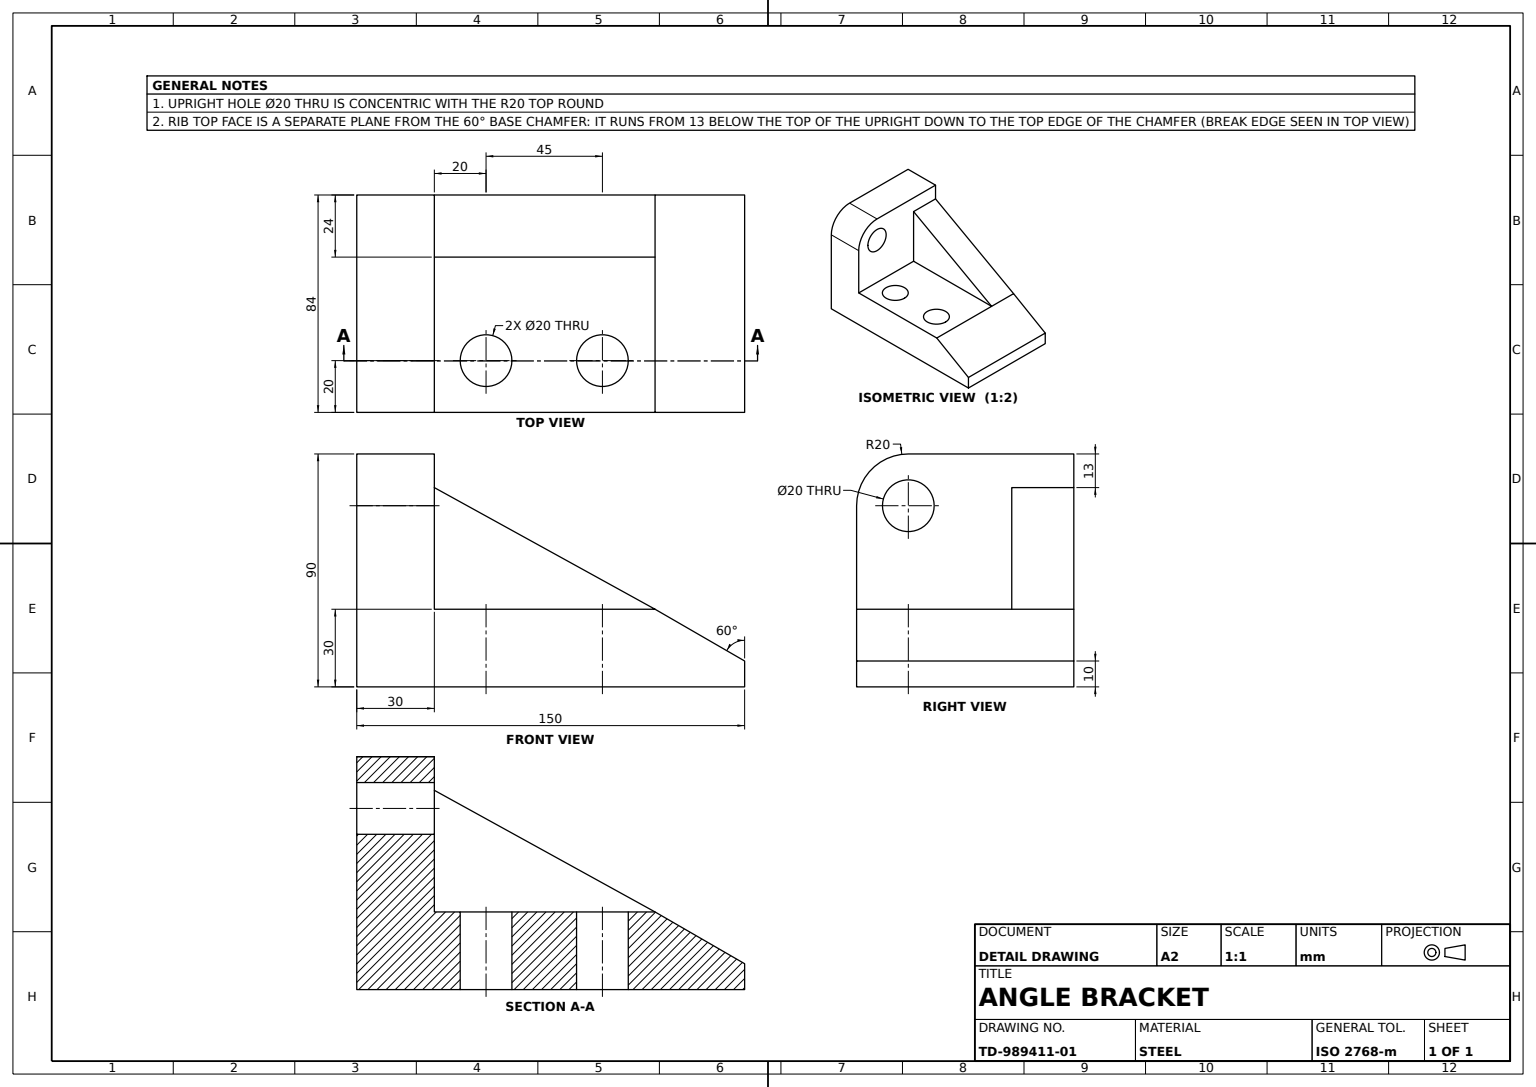
from build123d import *

# Parameters (mm, degrees)
BRACKET_BODY_DEPTH           = 42
UPRIGHT_TOP_ROUND_R20_R      = 20
SUPPORT_RIB_REACH            = 146.156
SUPPORT_RIB_SKETCH_WALL_W    = 387.75542236
SUPPORT_RIB_SKETCH_WALL_H    = 24
BASE_MOUNTING_HOLES_REACH    = 106.828
BASE_MOUNTING_HOLES_SKETCH_R = 10
UPRIGHT_HOLE_20_REACH        = 157.769
UPRIGHT_HOLE_SKETCH_R        = 10


with BuildPart() as part:
    # Bracket Profile Sketch → Bracket Body (new, symmetric)
    with BuildSketch(Plane.XY):
        Polygon((-75, 90), (-75, 0), (75, 0), (75, 10), (40.358983849, 30), (-45, 30), (-45, 90), align=None)
    extrude(amount=BRACKET_BODY_DEPTH, both=True)

    # Upright Top Round R20
    upright_top_round_r20_edges = [part.edges().sort_by_distance(p)[0] for p in [
        (-60, 90, 42),
    ]]
    fillet(upright_top_round_r20_edges, radius=UPRIGHT_TOP_ROUND_R20_R)

    # Support Rib Sketch wall → Support Rib (add, up to next)
    with BuildSketch(Plane(origin=(-2.320508076, 53.5, -42), x_dir=(-0.875988049468, 0.482332807497, 0), z_dir=(0.482332807497, 0.875988049468, 0)), mode=Mode.PRIVATE) as support_rib_sk1:
        with Locations((0, 12)):
            Rectangle(SUPPORT_RIB_SKETCH_WALL_W, SUPPORT_RIB_SKETCH_WALL_H)
    support_rib_tool1 = extrude(support_rib_sk1.sketch, amount=-SUPPORT_RIB_REACH, mode=Mode.PRIVATE) - part.part
    add(support_rib_tool1.solids().sort_by_distance((-2.320508076, 53.5, -42))[0])

    # Base Mounting Holes Sketch → Base Mounting Holes (cut, up to next)
    with BuildSketch(Plane(origin=(0, 30, 0), x_dir=(1, 0, 0), z_dir=(0, 1, 0)), mode=Mode.PRIVATE) as base_mounting_holes_sk1:
        with Locations(Location((-25, -22, 0), (0, 0, 180))):
            Circle(BASE_MOUNTING_HOLES_SKETCH_R)
    base_mounting_holes_tool1 = extrude(base_mounting_holes_sk1.sketch, amount=-BASE_MOUNTING_HOLES_REACH, mode=Mode.PRIVATE) & part.part
    # Base Mounting Holes Sketch → Base Mounting Holes (cut, up to next)
    with BuildSketch(Plane(origin=(0, 30, 0), x_dir=(1, 0, 0), z_dir=(0, 1, 0)), mode=Mode.PRIVATE) as base_mounting_holes_sk2:
        with Locations(Location((20, -22, 0), (0, 0, 180))):
            Circle(BASE_MOUNTING_HOLES_SKETCH_R)
    base_mounting_holes_tool2 = extrude(base_mounting_holes_sk2.sketch, amount=-BASE_MOUNTING_HOLES_REACH, mode=Mode.PRIVATE) & part.part
    add(base_mounting_holes_tool1.solids().sort_by_distance((-25, 30, 22))[0], mode=Mode.SUBTRACT)
    add(base_mounting_holes_tool2.solids().sort_by_distance((20, 30, 22))[0], mode=Mode.SUBTRACT)

    # Upright Hole Sketch → Upright Hole Ø20 (cut, up to next)
    with BuildSketch(Plane(origin=(-45, 0, 0), x_dir=(0, 0, -1), z_dir=(1, 0, 0)), mode=Mode.PRIVATE) as upright_hole_20_sk1:
        with Locations((-22, 70)):
            Circle(UPRIGHT_HOLE_SKETCH_R)
    upright_hole_20_tool1 = extrude(upright_hole_20_sk1.sketch, amount=-UPRIGHT_HOLE_20_REACH, mode=Mode.PRIVATE) & part.part
    add(upright_hole_20_tool1.solids().sort_by_distance((-45, 70, 22))[0], mode=Mode.SUBTRACT)


solid = part.part
